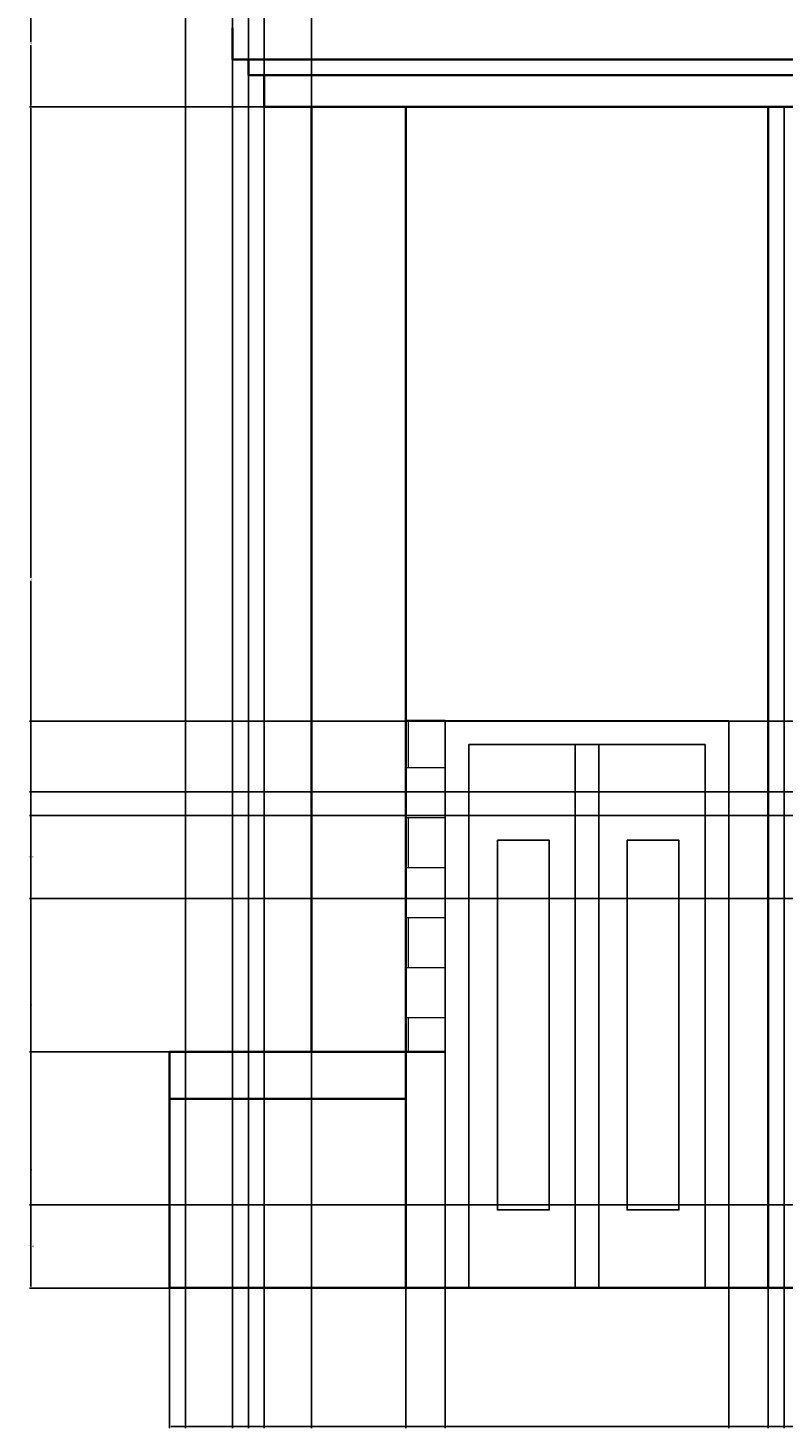
# Model space of a CAD drawing. Units: inches. Extents: x 2612 to 2948, y 481 to 865.
# Tile 1 of 7: x 2612 to 2708, y 481 to 659. Entities that reach past the tile are written whole.
import ezdxf

# ---------------------------------------------------------------- set-up
doc = ezdxf.new("R2010")
doc.units = ezdxf.units.IN
for name, color, linetype, lineweight in [('A-ANNO-DIMS', 2, 'Continuous', 18), ('A-COLS', 1, 'Continuous', 35), ('A-DOOR', 4, 'Continuous', 25), ('A-ELEV', 7, 'Continuous', 35), ('A-WALL-PATT', 8, 'Continuous', 13)]:
    doc.layers.add(name, color=color, linetype=linetype, lineweight=lineweight)
doc.styles.get("Standard").update_dxf_attribs({"font": 'arial.ttf'})
doc.dimstyles.get("Standard").update_dxf_attribs({"dimtxt": 0.18, "dimasz": 0.18, "dimexe": 0.18, "dimexo": 0.0625, "dimgap": 0.09, "dimtad": 0, "dimtih": 1, "dimtoh": 1, "dimdec": 4, "dimzin": 0, "dimdsep": 46, "dimtxsty": 'Standard', "dimcen": 0.09, "dimadec": 0, "dimazin": 0, "dimtfac": 1, "dimtdec": 4, "dimtofl": 0, "dimtmove": 0, "dimatfit": 3, "dimfxl": 1, "dimtolj": 1, "dimtzin": 0, "dimarcsym": 0})

# ---------------------------------------------------------------- blocks, each defined once
blk = doc.blocks.new('*D4')
at = {"layer": 'A-ANNO-DIMS', "color": 0, "lineweight": -2, "transparency": 16777216}
for p, q in [((2630.24, 529.04), (2612.53, 529.04)), ((2612.71, 528.86), (2612.71, 514.23)), ((2612.71, 499.22), (2612.71, 513.86)), ((2630.24, 499.04), (2612.53, 499.04))]:
    blk.add_line(p, q, dxfattribs=at)
at = {"layer": 'A-ANNO-DIMS', "color": 0, "transparency": 16777216}
for points in [[(2612.68, 528.86), (2612.74, 528.86), (2612.71, 529.04)], [(2612.68, 499.22), (2612.74, 499.22), (2612.71, 499.04)]]:
    blk.add_solid(points, dxfattribs=at)
at = {"layer": 'Defpoints', "color": 0, "transparency": 16777216}
for p in [(2612.71, 529.04), (2630.31, 529.04), (2630.31, 499.04)]:
    blk.add_point(p, dxfattribs=at)
at = {"layer": 'A-ANNO-DIMS', "color": 0, "transparency": 16777216, "insert": (2612.71, 514.04), "char_height": 0.18, "attachment_point": 5}
blk.add_mtext('\\A1;30', dxfattribs=at)
blk = doc.blocks.new('*D5')
at = {"layer": 'A-ANNO-DIMS', "color": 0, "lineweight": -2, "transparency": 16777216}
for p, q in [((2648.24, 649.04), (2612.53, 649.04)), ((2612.71, 648.86), (2612.71, 589.23)), ((2612.71, 529.22), (2612.71, 588.86)), ((2630.24, 529.04), (2612.53, 529.04))]:
    blk.add_line(p, q, dxfattribs=at)
at = {"layer": 'A-ANNO-DIMS', "color": 0, "transparency": 16777216}
for points in [[(2612.68, 648.86), (2612.74, 648.86), (2612.71, 649.04)], [(2612.68, 529.22), (2612.74, 529.22), (2612.71, 529.04)]]:
    blk.add_solid(points, dxfattribs=at)
at = {"layer": 'Defpoints', "color": 0, "transparency": 16777216}
for p in [(2612.71, 649.04), (2648.31, 649.04), (2630.31, 529.04)]:
    blk.add_point(p, dxfattribs=at)
at = {"layer": 'A-ANNO-DIMS', "color": 0, "transparency": 16777216, "insert": (2612.71, 589.04), "char_height": 0.18, "attachment_point": 5}
blk.add_mtext('\\A1;120', dxfattribs=at)
blk = doc.blocks.new('*D6')
at = {"layer": 'A-ANNO-DIMS', "color": 0, "lineweight": -2, "transparency": 16777216}
for p, q in [((2630.24, 665.04), (2612.53, 665.04)), ((2612.71, 664.86), (2612.71, 657.23)), ((2612.71, 649.22), (2612.71, 656.86)), ((2648.24, 649.04), (2612.53, 649.04))]:
    blk.add_line(p, q, dxfattribs=at)
at = {"layer": 'A-ANNO-DIMS', "color": 0, "transparency": 16777216}
for points in [[(2612.68, 664.86), (2612.74, 664.86), (2612.71, 665.04)], [(2612.68, 649.22), (2612.74, 649.22), (2612.71, 649.04)]]:
    blk.add_solid(points, dxfattribs=at)
at = {"layer": 'Defpoints', "color": 0, "transparency": 16777216}
for p in [(2612.71, 665.04), (2630.31, 665.04), (2648.31, 649.04)]:
    blk.add_point(p, dxfattribs=at)
at = {"layer": 'A-ANNO-DIMS', "color": 0, "transparency": 16777216, "insert": (2612.71, 657.04), "char_height": 0.18, "attachment_point": 5}
blk.add_mtext('\\A1;16', dxfattribs=at)
blk = doc.blocks.new('*D16')
at = {"layer": 'A-ANNO-DIMS', "color": 0, "lineweight": -2, "transparency": 16777216}
for p, q in [((2648.31, 528.98), (2648.31, 481.26)), ((2630.31, 498.98), (2630.31, 481.26)), ((2630.49, 481.44), (2639.1, 481.44)), ((2648.13, 481.44), (2639.52, 481.44))]:
    blk.add_line(p, q, dxfattribs=at)
at = {"layer": 'A-ANNO-DIMS', "color": 0, "transparency": 16777216}
for points in [[(2630.49, 481.47), (2630.49, 481.41), (2630.31, 481.44)], [(2648.13, 481.47), (2648.13, 481.41), (2648.31, 481.44)]]:
    blk.add_solid(points, dxfattribs=at)
at = {"layer": 'Defpoints', "color": 0, "transparency": 16777216}
for p in [(2648.31, 529.04), (2630.31, 499.04), (2648.31, 481.44)]:
    blk.add_point(p, dxfattribs=at)
at = {"layer": 'A-ANNO-DIMS', "color": 0, "transparency": 16777216, "insert": (2639.31, 481.44), "char_height": 0.18, "attachment_point": 5}
blk.add_mtext('\\A1;18', dxfattribs=at)
blk = doc.blocks.new('*D17')
at = {"layer": 'A-ANNO-DIMS', "color": 0, "lineweight": -2, "transparency": 16777216}
for p, q in [((2648.31, 528.98), (2648.31, 481.26)), ((2660.31, 528.98), (2660.31, 481.26)), ((2648.49, 481.44), (2654.1, 481.44)), ((2660.13, 481.44), (2654.52, 481.44))]:
    blk.add_line(p, q, dxfattribs=at)
at = {"layer": 'A-ANNO-DIMS', "color": 0, "transparency": 16777216}
for points in [[(2648.49, 481.47), (2648.49, 481.41), (2648.31, 481.44)], [(2660.13, 481.47), (2660.13, 481.41), (2660.31, 481.44)]]:
    blk.add_solid(points, dxfattribs=at)
at = {"layer": 'Defpoints', "color": 0, "transparency": 16777216}
for p in [(2648.31, 529.04), (2660.31, 529.04), (2660.31, 481.44)]:
    blk.add_point(p, dxfattribs=at)
at = {"layer": 'A-ANNO-DIMS', "color": 0, "transparency": 16777216, "insert": (2654.31, 481.44), "char_height": 0.18, "attachment_point": 5}
blk.add_mtext('\\A1;12', dxfattribs=at)
blk = doc.blocks.new('*D18')
at = {"layer": 'A-ANNO-DIMS', "color": 0, "lineweight": -2, "transparency": 16777216}
for p, q in [((2665.31, 570.98), (2665.31, 481.26)), ((2660.31, 528.98), (2660.31, 481.26)), ((2660.49, 481.44), (2662.66, 481.44)), ((2665.13, 481.44), (2662.96, 481.44))]:
    blk.add_line(p, q, dxfattribs=at)
at = {"layer": 'A-ANNO-DIMS', "color": 0, "transparency": 16777216}
for points in [[(2660.49, 481.47), (2660.49, 481.41), (2660.31, 481.44)], [(2665.13, 481.47), (2665.13, 481.41), (2665.31, 481.44)]]:
    blk.add_solid(points, dxfattribs=at)
at = {"layer": 'Defpoints', "color": 0, "transparency": 16777216}
for p in [(2665.31, 571.04), (2660.31, 529.04), (2665.31, 481.44)]:
    blk.add_point(p, dxfattribs=at)
at = {"layer": 'A-ANNO-DIMS', "color": 0, "transparency": 16777216, "insert": (2662.81, 481.44), "char_height": 0.18, "attachment_point": 5}
blk.add_mtext('\\A1;5', dxfattribs=at)
blk = doc.blocks.new('*D19')
at = {"layer": 'A-ANNO-DIMS', "color": 0, "lineweight": -2, "transparency": 16777216}
for p, q in [((2665.31, 570.98), (2665.31, 481.26)), ((2701.31, 570.98), (2701.31, 481.26)), ((2665.49, 481.44), (2683.09, 481.44)), ((2701.13, 481.44), (2683.53, 481.44))]:
    blk.add_line(p, q, dxfattribs=at)
at = {"layer": 'A-ANNO-DIMS', "color": 0, "transparency": 16777216}
for points in [[(2665.49, 481.47), (2665.49, 481.41), (2665.31, 481.44)], [(2701.13, 481.47), (2701.13, 481.41), (2701.31, 481.44)]]:
    blk.add_solid(points, dxfattribs=at)
at = {"layer": 'Defpoints', "color": 0, "transparency": 16777216}
for p in [(2665.31, 571.04), (2701.31, 571.04), (2701.31, 481.44)]:
    blk.add_point(p, dxfattribs=at)
at = {"layer": 'A-ANNO-DIMS', "color": 0, "transparency": 16777216, "insert": (2683.31, 481.44), "char_height": 0.18, "attachment_point": 5}
blk.add_mtext('\\A1;36', dxfattribs=at)
blk = doc.blocks.new('*D20')
at = {"layer": 'A-ANNO-DIMS', "color": 0, "lineweight": -2, "transparency": 16777216}
for p, q in [((2706.31, 648.98), (2706.31, 481.26)), ((2701.31, 570.98), (2701.31, 481.26)), ((2701.49, 481.44), (2703.66, 481.44)), ((2706.13, 481.44), (2703.96, 481.44))]:
    blk.add_line(p, q, dxfattribs=at)
at = {"layer": 'A-ANNO-DIMS', "color": 0, "transparency": 16777216}
for points in [[(2701.49, 481.47), (2701.49, 481.41), (2701.31, 481.44)], [(2706.13, 481.47), (2706.13, 481.41), (2706.31, 481.44)]]:
    blk.add_solid(points, dxfattribs=at)
at = {"layer": 'Defpoints', "color": 0, "transparency": 16777216}
for p in [(2706.31, 649.04), (2701.31, 571.04), (2706.31, 481.44)]:
    blk.add_point(p, dxfattribs=at)
at = {"layer": 'A-ANNO-DIMS', "color": 0, "transparency": 16777216, "insert": (2703.81, 481.44), "char_height": 0.18, "attachment_point": 5}
blk.add_mtext('\\A1;5', dxfattribs=at)
blk = doc.blocks.new('*D21')
at = {"layer": 'A-ANNO-DIMS', "color": 0, "lineweight": -2, "transparency": 16777216}
for p, q in [((2706.31, 648.98), (2706.31, 481.26)), ((2708.31, 648.98), (2708.31, 481.26)), ((2706.49, 481.44), (2707.16, 481.44)), ((2708.13, 481.44), (2707.46, 481.44))]:
    blk.add_line(p, q, dxfattribs=at)
at = {"layer": 'A-ANNO-DIMS', "color": 0, "transparency": 16777216}
for points in [[(2706.49, 481.47), (2706.49, 481.41), (2706.31, 481.44)], [(2708.13, 481.47), (2708.13, 481.41), (2708.31, 481.44)]]:
    blk.add_solid(points, dxfattribs=at)
at = {"layer": 'Defpoints', "color": 0, "transparency": 16777216}
for p in [(2706.31, 649.04), (2708.31, 649.04), (2708.31, 481.44)]:
    blk.add_point(p, dxfattribs=at)
at = {"layer": 'A-ANNO-DIMS', "color": 0, "transparency": 16777216, "insert": (2707.31, 481.44), "char_height": 0.18, "attachment_point": 5}
blk.add_mtext('\\A1;2', dxfattribs=at)
blk = doc.blocks.new('*D22')
at = {"layer": 'A-ANNO-DIMS', "color": 0, "lineweight": -2, "transparency": 16777216}
for p, q in [((2708.31, 648.98), (2708.31, 481.26)), ((2831.31, 570.98), (2831.31, 481.26)), ((2708.49, 481.44), (2769.53, 481.44)), ((2831.13, 481.44), (2770.09, 481.44))]:
    blk.add_line(p, q, dxfattribs=at)
at = {"layer": 'A-ANNO-DIMS', "color": 0, "transparency": 16777216}
for points in [[(2708.49, 481.47), (2708.49, 481.41), (2708.31, 481.44)], [(2831.13, 481.47), (2831.13, 481.41), (2831.31, 481.44)]]:
    blk.add_solid(points, dxfattribs=at)
at = {"layer": 'Defpoints', "color": 0, "transparency": 16777216}
for p in [(2708.31, 649.04), (2831.31, 571.04), (2831.31, 481.44)]:
    blk.add_point(p, dxfattribs=at)
at = {"layer": 'A-ANNO-DIMS', "color": 0, "transparency": 16777216, "insert": (2769.81, 481.44), "char_height": 0.18, "attachment_point": 5}
blk.add_mtext('\\A1;123', dxfattribs=at)
blk = doc.blocks.new('*D39')
at = {"layer": 'A-ANNO-DIMS', "color": 0, "lineweight": -2, "transparency": 16777216}
for p, q in [((2665.24, 571.04), (2612.53, 571.04)), ((2612.71, 570.86), (2612.71, 535.22)), ((2612.71, 499.22), (2612.71, 534.86)), ((2665.24, 499.04), (2612.53, 499.04))]:
    blk.add_line(p, q, dxfattribs=at)
at = {"layer": 'A-ANNO-DIMS', "color": 0, "transparency": 16777216}
for points in [[(2612.68, 570.86), (2612.74, 570.86), (2612.71, 571.04)], [(2612.68, 499.22), (2612.74, 499.22), (2612.71, 499.04)]]:
    blk.add_solid(points, dxfattribs=at)
at = {"layer": 'Defpoints', "color": 0, "transparency": 16777216}
for p in [(2665.31, 571.04), (2612.71, 499.04), (2665.31, 499.04)]:
    blk.add_point(p, dxfattribs=at)
at = {"layer": 'A-ANNO-DIMS', "color": 0, "transparency": 16777216, "insert": (2612.71, 535.04), "char_height": 0.18, "attachment_point": 5}
blk.add_mtext('\\A1;72', dxfattribs=at)
blk = doc.blocks.new('*D41')
at = {"layer": 'A-ANNO-DIMS', "color": 0, "lineweight": -2, "transparency": 16777216}
for p, q in [((2632.31, 802.98), (2632.31, 481.26)), ((2638.31, 792.98), (2638.31, 481.26)), ((2632.49, 481.44), (2635.16, 481.44)), ((2638.13, 481.44), (2635.46, 481.44))]:
    blk.add_line(p, q, dxfattribs=at)
at = {"layer": 'A-ANNO-DIMS', "color": 0, "transparency": 16777216}
for points in [[(2632.49, 481.47), (2632.49, 481.41), (2632.31, 481.44)], [(2638.13, 481.47), (2638.13, 481.41), (2638.31, 481.44)]]:
    blk.add_solid(points, dxfattribs=at)
at = {"layer": 'Defpoints', "color": 0, "transparency": 16777216}
for p in [(2632.31, 803.04), (2638.31, 793.04), (2638.31, 481.44)]:
    blk.add_point(p, dxfattribs=at)
at = {"layer": 'A-ANNO-DIMS', "color": 0, "transparency": 16777216, "insert": (2635.31, 481.44), "char_height": 0.18, "attachment_point": 5}
blk.add_mtext('\\A1;6', dxfattribs=at)
blk = doc.blocks.new('*D42')
at = {"layer": 'A-ANNO-DIMS', "color": 0, "lineweight": -2, "transparency": 16777216}
for p, q in [((2638.31, 792.98), (2638.31, 481.26)), ((2640.31, 790.98), (2640.31, 481.26)), ((2638.49, 481.44), (2639.16, 481.44)), ((2640.13, 481.44), (2639.46, 481.44))]:
    blk.add_line(p, q, dxfattribs=at)
at = {"layer": 'A-ANNO-DIMS', "color": 0, "transparency": 16777216}
for points in [[(2638.49, 481.47), (2638.49, 481.41), (2638.31, 481.44)], [(2640.13, 481.47), (2640.13, 481.41), (2640.31, 481.44)]]:
    blk.add_solid(points, dxfattribs=at)
at = {"layer": 'Defpoints', "color": 0, "transparency": 16777216}
for p in [(2638.31, 793.04), (2640.31, 791.04), (2640.31, 481.44)]:
    blk.add_point(p, dxfattribs=at)
at = {"layer": 'A-ANNO-DIMS', "color": 0, "transparency": 16777216, "insert": (2639.31, 481.44), "char_height": 0.18, "attachment_point": 5}
blk.add_mtext('\\A1;2', dxfattribs=at)
blk = doc.blocks.new('*D43')
at = {"layer": 'A-ANNO-DIMS', "color": 0, "lineweight": -2, "transparency": 16777216}
for p, q in [((2640.31, 790.98), (2640.31, 481.26)), ((2642.31, 786.98), (2642.31, 481.26)), ((2640.49, 481.44), (2641.16, 481.44)), ((2642.13, 481.44), (2641.46, 481.44))]:
    blk.add_line(p, q, dxfattribs=at)
at = {"layer": 'A-ANNO-DIMS', "color": 0, "transparency": 16777216}
for points in [[(2640.49, 481.47), (2640.49, 481.41), (2640.31, 481.44)], [(2642.13, 481.47), (2642.13, 481.41), (2642.31, 481.44)]]:
    blk.add_solid(points, dxfattribs=at)
at = {"layer": 'Defpoints', "color": 0, "transparency": 16777216}
for p in [(2640.31, 791.04), (2642.31, 787.04), (2642.31, 481.44)]:
    blk.add_point(p, dxfattribs=at)
at = {"layer": 'A-ANNO-DIMS', "color": 0, "transparency": 16777216, "insert": (2641.31, 481.44), "char_height": 0.18, "attachment_point": 5}
blk.add_mtext('\\A1;2', dxfattribs=at)
blk = doc.blocks.new('*D44')
at = {"layer": 'A-ANNO-DIMS', "color": 0, "lineweight": -2, "transparency": 16777216}
for p, q in [((2642.31, 786.98), (2642.31, 481.26)), ((2648.31, 786.98), (2648.31, 481.26)), ((2642.49, 481.44), (2645.16, 481.44)), ((2648.13, 481.44), (2645.46, 481.44))]:
    blk.add_line(p, q, dxfattribs=at)
at = {"layer": 'A-ANNO-DIMS', "color": 0, "transparency": 16777216}
for points in [[(2642.49, 481.47), (2642.49, 481.41), (2642.31, 481.44)], [(2648.13, 481.47), (2648.13, 481.41), (2648.31, 481.44)]]:
    blk.add_solid(points, dxfattribs=at)
at = {"layer": 'Defpoints', "color": 0, "transparency": 16777216}
for p in [(2642.31, 787.04), (2648.31, 787.04), (2648.31, 481.44)]:
    blk.add_point(p, dxfattribs=at)
at = {"layer": 'A-ANNO-DIMS', "color": 0, "transparency": 16777216, "insert": (2645.31, 481.44), "char_height": 0.18, "attachment_point": 5}
blk.add_mtext('\\A1;6', dxfattribs=at)
blk = doc.blocks.new('*D59')
at = {"layer": 'A-ANNO-DIMS', "color": 0, "lineweight": -2, "transparency": 16777216}
for p, q in [((2715.74, 509.59), (2612.53, 509.59)), ((2612.71, 509.41), (2612.71, 504.5)), ((2612.71, 499.22), (2612.71, 504.14)), ((2715.74, 499.04), (2612.53, 499.04))]:
    blk.add_line(p, q, dxfattribs=at)
at = {"layer": 'A-ANNO-DIMS', "color": 0, "transparency": 16777216}
for points in [[(2612.68, 509.41), (2612.74, 509.41), (2612.71, 509.59)], [(2612.68, 499.22), (2612.74, 499.22), (2612.71, 499.04)]]:
    blk.add_solid(points, dxfattribs=at)
at = {"layer": 'Defpoints', "color": 0, "transparency": 16777216}
for p in [(2612.71, 509.59), (2715.81, 509.59), (2715.81, 499.04)]:
    blk.add_point(p, dxfattribs=at)
at = {"layer": 'A-ANNO-DIMS', "color": 0, "transparency": 16777216, "insert": (2612.71, 504.32), "char_height": 0.18, "attachment_point": 5}
blk.add_mtext('\\A1;10.548', dxfattribs=at)
blk = doc.blocks.new('*D60')
at = {"layer": 'A-ANNO-DIMS', "color": 0, "lineweight": -2, "transparency": 16777216}
for p, q in [((2715.74, 548.5), (2612.53, 548.5)), ((2612.71, 548.32), (2612.71, 529.23)), ((2612.71, 509.77), (2612.71, 528.86)), ((2715.74, 509.59), (2612.53, 509.59))]:
    blk.add_line(p, q, dxfattribs=at)
at = {"layer": 'A-ANNO-DIMS', "color": 0, "transparency": 16777216}
for points in [[(2612.68, 548.32), (2612.74, 548.32), (2612.71, 548.5)], [(2612.68, 509.77), (2612.74, 509.77), (2612.71, 509.59)]]:
    blk.add_solid(points, dxfattribs=at)
at = {"layer": 'Defpoints', "color": 0, "transparency": 16777216}
for p in [(2612.71, 548.5), (2715.81, 548.5), (2715.81, 509.59)]:
    blk.add_point(p, dxfattribs=at)
at = {"layer": 'A-ANNO-DIMS', "color": 0, "transparency": 16777216, "insert": (2612.71, 529.04), "char_height": 0.18, "attachment_point": 5}
blk.add_mtext('\\A1;38.9', dxfattribs=at)
blk = doc.blocks.new('*D61')
at = {"layer": 'A-ANNO-DIMS', "color": 0, "lineweight": -2, "transparency": 16777216}
for p, q in [((2715.74, 559.04), (2612.53, 559.04)), ((2612.71, 558.86), (2612.71, 553.95)), ((2612.71, 548.68), (2612.71, 553.59)), ((2715.74, 548.5), (2612.53, 548.5))]:
    blk.add_line(p, q, dxfattribs=at)
at = {"layer": 'A-ANNO-DIMS', "color": 0, "transparency": 16777216}
for points in [[(2612.68, 558.86), (2612.74, 558.86), (2612.71, 559.04)], [(2612.68, 548.68), (2612.74, 548.68), (2612.71, 548.5)]]:
    blk.add_solid(points, dxfattribs=at)
at = {"layer": 'Defpoints', "color": 0, "transparency": 16777216}
for p in [(2612.71, 559.04), (2715.81, 559.04), (2715.81, 548.5)]:
    blk.add_point(p, dxfattribs=at)
at = {"layer": 'A-ANNO-DIMS', "color": 0, "transparency": 16777216, "insert": (2612.71, 553.77), "char_height": 0.18, "attachment_point": 5}
blk.add_mtext('\\A1;10.548', dxfattribs=at)
blk = doc.blocks.new('*D62')
at = {"layer": 'A-ANNO-DIMS', "color": 0, "lineweight": -2, "transparency": 16777216}
for p, q in [((2712.74, 562.04), (2612.53, 562.04)), ((2612.71, 561.86), (2612.71, 560.73)), ((2612.71, 559.22), (2612.71, 560.36)), ((2715.74, 559.04), (2612.53, 559.04))]:
    blk.add_line(p, q, dxfattribs=at)
at = {"layer": 'A-ANNO-DIMS', "color": 0, "transparency": 16777216}
for points in [[(2612.68, 561.86), (2612.74, 561.86), (2612.71, 562.04)], [(2612.68, 559.22), (2612.74, 559.22), (2612.71, 559.04)]]:
    blk.add_solid(points, dxfattribs=at)
at = {"layer": 'Defpoints', "color": 0, "transparency": 16777216}
for p in [(2612.71, 562.04), (2712.81, 562.04), (2715.81, 559.04)]:
    blk.add_point(p, dxfattribs=at)
at = {"layer": 'A-ANNO-DIMS', "color": 0, "transparency": 16777216, "insert": (2612.71, 560.54), "char_height": 0.18, "attachment_point": 5}
blk.add_mtext('\\A1;3', dxfattribs=at)
blk = doc.blocks.new('*D63')
at = {"layer": 'A-ANNO-DIMS', "color": 0, "lineweight": -2, "transparency": 16777216}
for p, q in [((2722.45, 571.04), (2612.53, 571.04)), ((2612.71, 570.86), (2612.71, 566.73)), ((2612.71, 562.22), (2612.71, 566.36)), ((2712.74, 562.04), (2612.53, 562.04))]:
    blk.add_line(p, q, dxfattribs=at)
at = {"layer": 'A-ANNO-DIMS', "color": 0, "transparency": 16777216}
for points in [[(2612.68, 570.86), (2612.74, 570.86), (2612.71, 571.04)], [(2612.68, 562.22), (2612.74, 562.22), (2612.71, 562.04)]]:
    blk.add_solid(points, dxfattribs=at)
at = {"layer": 'Defpoints', "color": 0, "transparency": 16777216}
for p in [(2612.71, 571.04), (2722.51, 571.04), (2712.81, 562.04)]:
    blk.add_point(p, dxfattribs=at)
at = {"layer": 'A-ANNO-DIMS', "color": 0, "transparency": 16777216, "insert": (2612.71, 566.54), "char_height": 0.18, "attachment_point": 5}
blk.add_mtext('\\A1;9', dxfattribs=at)
blk = doc.blocks.new('*D87')
at = {"layer": 'A-ANNO-DIMS', "color": 0, "lineweight": -2, "transparency": 16777216}
for p, q in [((2630.31, 498.98), (2630.31, 481.26)), ((2930.31, 498.98), (2930.31, 481.26)), ((2630.49, 481.44), (2780.02, 481.44)), ((2930.13, 481.44), (2780.6, 481.44))]:
    blk.add_line(p, q, dxfattribs=at)
at = {"layer": 'A-ANNO-DIMS', "color": 0, "transparency": 16777216}
for points in [[(2630.49, 481.47), (2630.49, 481.41), (2630.31, 481.44)], [(2930.13, 481.47), (2930.13, 481.41), (2930.31, 481.44)]]:
    blk.add_solid(points, dxfattribs=at)
at = {"layer": 'Defpoints', "color": 0, "transparency": 16777216}
for p in [(2630.31, 499.04), (2930.31, 499.04), (2930.31, 481.44)]:
    blk.add_point(p, dxfattribs=at)
at = {"layer": 'A-ANNO-DIMS', "color": 0, "transparency": 16777216, "insert": (2780.31, 481.44), "char_height": 0.18, "attachment_point": 5}
blk.add_mtext('\\A1;300', dxfattribs=at)

msp = doc.modelspace()

# ---------------------------------------------------------------- hatches: boundary and pattern name
at = {"layer": 'A-WALL-PATT'}
h = msp.add_hatch(dxfattribs=at)
h.set_pattern_fill('BRICK', color=256)
h.paths.add_polyline_path([(2665.3074, 571.0443), (2660.3074, 571.0443), (2660.3074, 529.0443), (2665.3074, 529.0443)])

# ---------------------------------------------------------------- linework, layer by layer
at = {"layer": 'A-COLS'}
for p, q in [((2648.3074, 529.0443), (2648.3074, 649.0443)), ((2660.3074, 499.0443), (2660.3074, 649.0443))]:
    msp.add_line(p, q, dxfattribs=at)
at = {"layer": 'A-DOOR'}
for p, q in [((2665.3074, 499.0443), (2665.3074, 571.0443)), ((2665.3074, 571.0443), (2701.3074, 571.0443)), ((2665.3074, 571.0443), (2701.3074, 571.0443)), ((2701.3074, 499.0443), (2701.3074, 571.0443)), ((2668.3074, 499.0443), (2668.3074, 568.0443)), ((2668.3074, 568.0443), (2698.3074, 568.0443)), ((2681.8074, 568.0443), (2681.8074, 499.0443)), ((2684.8074, 568.0443), (2684.8074, 499.0443)), ((2698.3074, 499.0443), (2698.3074, 568.0443))]:
    msp.add_line(p, q, dxfattribs=at)
for points in [[(2671.9254, 555.8913), (2678.5069, 555.8913), (2678.5069, 508.9679), (2671.9254, 508.9679)], [(2688.3792, 555.8913), (2694.9607, 555.8913), (2694.9607, 508.9679), (2688.3792, 508.9679)]]:
    msp.add_lwpolyline(points, close=True, dxfattribs=at)
at = {"layer": 'A-ELEV'}
for p, q in [((2638.3074, 655.0443), (2638.3074, 659.0443)), ((2640.3074, 655.0443), (2638.3074, 655.0443)), ((2642.3074, 655.0443), (2640.3074, 655.0443)), ((2640.3074, 653.0443), (2640.3074, 655.0443)), ((2642.3074, 655.0443), (2918.3074, 655.0443)), ((2642.3074, 653.0443), (2640.3074, 653.0443)), ((2642.3074, 649.0443), (2642.3074, 653.0443)), ((2642.3074, 653.0443), (2918.3074, 653.0443)), ((2642.3074, 649.0443), (2918.3074, 649.0443)), ((2706.3074, 499.0443), (2706.3074, 649.0443)), ((2660.3074, 571.0443), (2665.3074, 571.0443)), ((2630.3074, 529.0443), (2660.3074, 529.0443)), ((2630.3074, 499.0443), (2630.3074, 529.0443)), ((2660.3074, 529.0443), (2665.3074, 529.0443)), ((2630.3074, 523.0443), (2660.3074, 523.0443)), ((2630.3074, 499.0443), (2930.3074, 499.0443))]:
    msp.add_line(p, q, dxfattribs=at)

# ---------------------------------------------------------------- dimensions: what is measured, and where the dimension line sits
at = {"layer": 'A-ANNO-DIMS'}
for base, p1, p2, picture, middle in [((2638.3074, 481.4443), (2632.3074, 803.0443), (2638.3074, 793.0443), '*D41', (2635.3074, 481.4443)), ((2640.3074, 481.4443), (2638.3074, 793.0443), (2640.3074, 791.0443), '*D42', (2639.3074, 481.4443)), ((2642.3074, 481.4443), (2640.3074, 791.0443), (2642.3074, 787.0443), '*D43', (2641.3074, 481.4443)), ((2648.3074, 481.4443), (2642.3074, 787.0443), (2648.3074, 787.0443), '*D44', (2645.3074, 481.4443)), ((2706.3074, 481.4443), (2701.3074, 571.0443), (2706.3074, 649.0443), '*D20', (2703.8074, 481.4443)), ((2708.3074, 481.4443), (2706.3074, 649.0443), (2708.3074, 649.0443), '*D21', (2707.3074, 481.4443)), ((2831.3074, 481.4443), (2708.3074, 649.0443), (2831.3074, 571.0443), '*D22', (2769.8074, 481.4443)), ((2665.3074, 481.4443), (2660.3074, 529.0443), (2665.3074, 571.0443), '*D18', (2662.8074, 481.4443)), ((2701.3074, 481.4443), (2665.3074, 571.0443), (2701.3074, 571.0443), '*D19', (2683.3074, 481.4443)), ((2648.3074, 481.4443), (2630.3074, 499.0443), (2648.3074, 529.0443), '*D16', (2639.3074, 481.4443)), ((2660.3074, 481.4443), (2648.3074, 529.0443), (2660.3074, 529.0443), '*D17', (2654.3074, 481.4443)), ((2930.3074, 481.4443), (2630.3074, 499.0443), (2930.3074, 499.0443), '*D87', (2780.3074, 481.4443))]:
    dim = msp.add_linear_dim(base=base, p1=p1, p2=p2, dimstyle='Standard', override={"dimdec": 0, "dimlfac": 1, "dimrnd": 0, "dimzin": 0, "dimdsep": 46, "dimlunit": 2}, dxfattribs=at)
    dim.commit()
    dim.dimension.update_dxf_attribs({"geometry": picture, "text_midpoint": middle})
for base, p1, p2, override, picture, middle in [((2612.7074, 665.0443), (2648.3074, 649.0443), (2630.3074, 665.0443), {"dimdec": 0, "dimlfac": 1, "dimrnd": 0, "dimzin": 0, "dimdsep": 46, "dimlunit": 2}, '*D6', (2612.7074, 657.0443)), ((2612.7074, 649.0443), (2630.3074, 529.0443), (2648.3074, 649.0443), {"dimdec": 0, "dimlfac": 1, "dimrnd": 0, "dimzin": 0, "dimdsep": 46, "dimlunit": 2}, '*D5', (2612.7074, 589.0443)), ((2612.7074, 499.0443), (2665.3074, 571.0443), (2665.3074, 499.0443), {"dimdec": 0, "dimlfac": 1, "dimrnd": 0, "dimzin": 0, "dimdsep": 46, "dimlunit": 2}, '*D39', (2612.7074, 535.0443)), ((2612.7074, 571.0443), (2712.8074, 562.0443), (2722.5147, 571.0443), {"dimdec": 0, "dimlfac": 1, "dimrnd": 0, "dimzin": 0, "dimdsep": 46, "dimlunit": 2}, '*D63', (2612.7074, 566.5443)), ((2612.7074, 562.0443), (2715.8074, 559.0443), (2712.8074, 562.0443), {"dimdec": 0, "dimlfac": 1, "dimrnd": 0, "dimzin": 0, "dimdsep": 46, "dimlunit": 2}, '*D62', (2612.7074, 560.5443)), ((2612.7074, 559.0443), (2715.8074, 548.4959), (2715.8074, 559.0443), {"dimdec": 3, "dimlfac": 1, "dimrnd": 0, "dimzin": 0, "dimdsep": 46, "dimlunit": 2}, '*D61', (2612.7074, 553.7701)), ((2612.7074, 548.4959), (2715.8074, 509.5927), (2715.8074, 548.4959), {"dimdec": 1, "dimlfac": 1, "dimrnd": 0, "dimzin": 0, "dimdsep": 46, "dimlunit": 2}, '*D60', (2612.7074, 529.0443)), ((2612.7074, 529.0443), (2630.3074, 499.0443), (2630.3074, 529.0443), {"dimdec": 0, "dimlfac": 1, "dimrnd": 0, "dimzin": 0, "dimdsep": 46, "dimlunit": 2}, '*D4', (2612.7074, 514.0443)), ((2612.7074, 509.5927), (2715.8074, 499.0443), (2715.8074, 509.5927), {"dimdec": 3, "dimlfac": 1, "dimrnd": 0, "dimzin": 0, "dimdsep": 46, "dimlunit": 2}, '*D59', (2612.7074, 504.3185))]:
    dim = msp.add_linear_dim(base=base, p1=p1, p2=p2, angle=90, dimstyle='Standard', override=override, dxfattribs=at)
    dim.commit()
    dim.dimension.update_dxf_attribs({"geometry": picture, "text_midpoint": middle})

doc.saveas('drawing.dxf')
